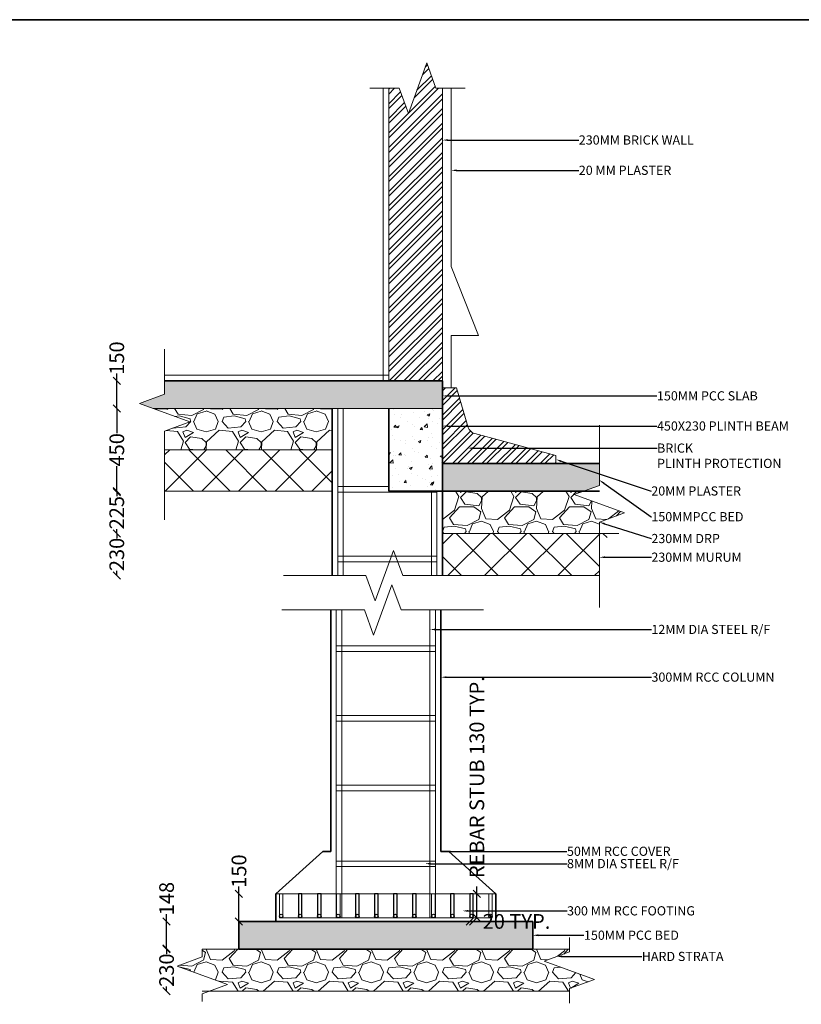
# Model space of a CAD drawing. Units: millimetres. Extents: x -6233 to 6805, y -5269 to 4890.
# Tile 3 of 4: x -1936 to 2321, y -472 to 4890. Entities that reach past the tile are written whole.
import ezdxf
from ezdxf import colors
from ezdxf.entities.mleader import LeaderData, LeaderLine
from ezdxf.math import Vec2, Vec3

# ---------------------------------------------------------------- set-up
doc = ezdxf.new("R2010")
doc.units = ezdxf.units.MM
doc.header["$MEASUREMENT"] = 0
for name, color, linetype, lineweight in [('S-ANNO-DIMS', 2, 'Continuous', 18), ('S-ANNO-TEXT', 3, 'Continuous', 18), ('S-ANNO-TTLB', 7, 'Continuous', 35), ('S-CONC', 7, 'Continuous', 35), ('S-FNDN', 8, 'Continuous', 18), ('S-PATT', 252, 'Continuous', 13), ('S-REIN', 1, 'Continuous', 25)]:
    doc.layers.add(name, color=color, linetype=linetype, lineweight=lineweight)
doc.styles.get("Standard").update_dxf_attribs({"font": 'arial.ttf'})
doc.dimstyles.get("Standard").update_dxf_attribs({"dimtxt": 80, "dimasz": 40, "dimexe": 0.18, "dimexo": 0.0625, "dimgap": 0.09, "dimtad": 0, "dimdec": 0, "dimzin": 0, "dimdsep": 46, "dimtxsty": 'Standard', "dimblk": 'OBLIQUE', "dimcen": 0.09, "dimadec": 0, "dimazin": 0, "dimtfac": 1, "dimtdec": 0, "dimtofl": 0, "dimtmove": 0, "dimatfit": 3, "dimfxl": 1, "dimfxlon": 1, "dimtolj": 1, "dimtzin": 0, "dimarcsym": 0})

# ---------------------------------------------------------------- blocks, each defined once
blk = doc.blocks.new('_Oblique')
at = {"color": 0, "linetype": 'ByBlock', "lineweight": -2}
blk.add_line((-0.5, -0.5), (0.5, 0.5), dxfattribs=at)
blk = doc.blocks.new('*D10')
at = {"layer": 'DEFPOINTS', "color": 0, "transparency": 16777216}
for p in [(-1136.3, -171.5), (-906.1, -171.5), (-906.1, -401.5)]:
    blk.add_point(p, dxfattribs=at)
at = {"layer": 'S-ANNO-DIMS', "color": 0, "lineweight": -2, "transparency": 16777216}
for p, q in [((-1135.3, -171.5), (-1136.5, -171.5)), ((-1136.3, -171.5), (-1136.3, -197.5)), ((-1135.3, -401.5), (-1136.5, -401.5)), ((-1136.3, -401.5), (-1136.3, -375.5))]:
    blk.add_line(p, q, dxfattribs=at)
at = {"layer": 'S-ANNO-DIMS', "color": 0, "lineweight": -2, "transparency": 16777216, "xscale": 40, "yscale": 40, "zscale": 40}
for p, rotation in [((-1136.3, -171.5), 90), ((-1136.3, -401.5), 270)]:
    blk.add_blockref('_Oblique', p, dxfattribs=dict(at, rotation=rotation))
at = {"layer": 'S-ANNO-DIMS', "color": 0, "transparency": 16777216, "insert": (-1136.3, -286.5), "char_height": 80, "attachment_point": 5, "rotation": 90}
blk.add_mtext('\\A1;230', dxfattribs=at)
blk = doc.blocks.new('*D11')
at = {"layer": 'DEFPOINTS', "color": 0, "transparency": 16777216}
for p in [(-1136.3, -21.5), (-742, -21.5), (-742, -169.1)]:
    blk.add_point(p, dxfattribs=at)
at = {"layer": 'S-ANNO-DIMS', "color": 0, "lineweight": -2, "transparency": 16777216}
for p, q in [((-1136.3, -21.5), (-1136.3, 18.5)), ((-1135.3, -21.5), (-1136.5, -21.5)), ((-1136.3, -169.1), (-1136.3, -21.5)), ((-1135.3, -169.1), (-1136.5, -169.1))]:
    blk.add_line(p, q, dxfattribs=at)
at = {"layer": 'S-ANNO-DIMS', "color": 0, "lineweight": -2, "transparency": 16777216, "xscale": 40, "yscale": 40, "zscale": 40}
for p, rotation in [((-1136.3, -21.5), 90), ((-1136.3, -169.1), 270)]:
    blk.add_blockref('_Oblique', p, dxfattribs=dict(at, rotation=rotation))
at = {"layer": 'S-ANNO-DIMS', "color": 0, "transparency": 16777216, "insert": (-1136.3, 103.3), "char_height": 80, "attachment_point": 5, "rotation": 90}
blk.add_mtext('\\A1;148', dxfattribs=at)
blk = doc.blocks.new('*D12')
at = {"layer": 'DEFPOINTS', "color": 0, "transparency": 16777216}
for p in [(-742, 128.5), (-542, 128.5), (-542, -21.5)]:
    blk.add_point(p, dxfattribs=at)
at = {"layer": 'S-ANNO-DIMS', "color": 0, "lineweight": -2, "transparency": 16777216}
for p, q in [((-742, 128.5), (-742, 168.5)), ((-741, 128.5), (-742.2, 128.5)), ((-742, -21.5), (-742, 128.5)), ((-741, -21.5), (-742.2, -21.5))]:
    blk.add_line(p, q, dxfattribs=at)
at = {"layer": 'S-ANNO-DIMS', "color": 0, "lineweight": -2, "transparency": 16777216, "xscale": 40, "yscale": 40, "zscale": 40}
for p, rotation in [((-742, 128.5), 90), ((-742, -21.5), 270)]:
    blk.add_blockref('_Oblique', p, dxfattribs=dict(at, rotation=rotation))
at = {"layer": 'S-ANNO-DIMS', "color": 0, "transparency": 16777216, "insert": (-742, 253.1), "char_height": 80, "attachment_point": 5, "rotation": 90}
blk.add_mtext('\\A1;150', dxfattribs=at)
blk = doc.blocks.new('*D13')
at = {"layer": 'DEFPOINTS', "color": 0, "transparency": 16777216}
for p in [(-1407.6, 2092.6), (374.4, 2092.6), (374.4, 1862.6)]:
    blk.add_point(p, dxfattribs=at)
at = {"layer": 'S-ANNO-DIMS', "color": 0, "lineweight": -2, "transparency": 16777216}
for p, q in [((-1406.6, 2092.6), (-1407.8, 2092.6)), ((-1407.6, 2092.6), (-1407.6, 2066.7)), ((-1407.6, 1862.6), (-1407.6, 1888.6)), ((-1406.6, 1862.6), (-1407.8, 1862.6))]:
    blk.add_line(p, q, dxfattribs=at)
at = {"layer": 'S-ANNO-DIMS', "color": 0, "lineweight": -2, "transparency": 16777216, "xscale": 40, "yscale": 40, "zscale": 40}
for p, rotation in [((-1407.6, 2092.6), 90), ((-1407.6, 1862.6), 270)]:
    blk.add_blockref('_Oblique', p, dxfattribs=dict(at, rotation=rotation))
at = {"layer": 'S-ANNO-DIMS', "color": 0, "transparency": 16777216, "insert": (-1407.6, 1977.6), "char_height": 80, "attachment_point": 5, "rotation": 90}
blk.add_mtext('\\A1;230', dxfattribs=at)
blk = doc.blocks.new('*D14')
at = {"layer": 'DEFPOINTS', "color": 0, "transparency": 16777216}
for p in [(-1407.8, 2317.5), (366.2, 2317.5), (366.2, 2092.6)]:
    blk.add_point(p, dxfattribs=at)
at = {"layer": 'S-ANNO-DIMS', "color": 0, "lineweight": -2, "transparency": 16777216}
for p, q in [((-1406.8, 2317.5), (-1408, 2317.5)), ((-1407.8, 2317.5), (-1407.8, 2294.5)), ((-1406.8, 2092.6), (-1408, 2092.6)), ((-1407.8, 2092.6), (-1407.8, 2115.6))]:
    blk.add_line(p, q, dxfattribs=at)
at = {"layer": 'S-ANNO-DIMS', "color": 0, "lineweight": -2, "transparency": 16777216, "xscale": 40, "yscale": 40, "zscale": 40}
for p, rotation in [((-1407.8, 2317.5), 90), ((-1407.8, 2092.6), 270)]:
    blk.add_blockref('_Oblique', p, dxfattribs=dict(at, rotation=rotation))
at = {"layer": 'S-ANNO-DIMS', "color": 0, "transparency": 16777216, "insert": (-1407.8, 2205), "char_height": 80, "attachment_point": 5, "rotation": 90}
blk.add_mtext('\\A1;225', dxfattribs=at)
blk = doc.blocks.new('*D15')
at = {"layer": 'DEFPOINTS', "color": 0, "transparency": 16777216}
for p in [(-1407.4, 2772.6), (-1147, 2772.6), (-1147, 2322.6)]:
    blk.add_point(p, dxfattribs=at)
at = {"layer": 'S-ANNO-DIMS', "color": 0, "lineweight": -2, "transparency": 16777216}
for p, q in [((-1406.4, 2772.6), (-1407.6, 2772.6)), ((-1407.4, 2772.6), (-1407.4, 2637.6)), ((-1407.4, 2322.6), (-1407.4, 2457.7)), ((-1406.4, 2322.6), (-1407.6, 2322.6))]:
    blk.add_line(p, q, dxfattribs=at)
at = {"layer": 'S-ANNO-DIMS', "color": 0, "lineweight": -2, "transparency": 16777216, "xscale": 40, "yscale": 40, "zscale": 40}
for p, rotation in [((-1407.4, 2772.6), 90), ((-1407.4, 2322.6), 270)]:
    blk.add_blockref('_Oblique', p, dxfattribs=dict(at, rotation=rotation))
at = {"layer": 'S-ANNO-DIMS', "color": 0, "transparency": 16777216, "insert": (-1407.4, 2547.6), "char_height": 80, "attachment_point": 5, "rotation": 90}
blk.add_mtext('\\A1;450', dxfattribs=at)
blk = doc.blocks.new('*D16')
at = {"layer": 'DEFPOINTS', "color": 0, "transparency": 16777216}
for p in [(-1407.6, 2922.6), (-1113.4, 2922.6), (-1113.4, 2772.6)]:
    blk.add_point(p, dxfattribs=at)
at = {"layer": 'S-ANNO-DIMS', "color": 0, "lineweight": -2, "transparency": 16777216}
for p, q in [((-1407.6, 2922.6), (-1407.6, 2962.6)), ((-1406.6, 2922.6), (-1407.8, 2922.6)), ((-1407.6, 2772.6), (-1407.6, 2922.6)), ((-1406.6, 2772.6), (-1407.8, 2772.6))]:
    blk.add_line(p, q, dxfattribs=at)
at = {"layer": 'S-ANNO-DIMS', "color": 0, "lineweight": -2, "transparency": 16777216, "xscale": 40, "yscale": 40, "zscale": 40}
for p, rotation in [((-1407.6, 2922.6), 90), ((-1407.6, 2772.6), 270)]:
    blk.add_blockref('_Oblique', p, dxfattribs=dict(at, rotation=rotation))
at = {"layer": 'S-ANNO-DIMS', "color": 0, "transparency": 16777216, "insert": (-1407.6, 3047.2), "char_height": 80, "attachment_point": 5, "rotation": 90}
blk.add_mtext('\\A1;150', dxfattribs=at)
blk = doc.blocks.new('REBAR-STUB-TRAP')
for p, q in [((0, 130), (0, 32.5)), ((19.5, 130), (0, 130)), ((19.5, 0), (19.5, 130)), ((0, 32.5), (0, 0))]:
    blk.add_line(p, q)
blk = doc.blocks.new('*D30')
at = {"layer": 'DEFPOINTS', "color": 0, "transparency": 16777216}
for p in [(534.3, 128.5), (553.8, 128.5), (534.3, -1.5)]:
    blk.add_point(p, dxfattribs=at)
at = {"layer": 'S-ANNO-DIMS', "color": 0, "lineweight": -2, "transparency": 16777216}
for p, q in [((553.8, 128.5), (553.8, 168.5)), ((552.8, 128.5), (554, 128.5)), ((553.8, -1.5), (553.8, 128.5)), ((552.8, -1.5), (554, -1.5))]:
    blk.add_line(p, q, dxfattribs=at)
at = {"layer": 'S-ANNO-DIMS', "color": 0, "lineweight": -2, "transparency": 16777216, "xscale": 40, "yscale": 40, "zscale": 40}
for p, rotation in [((553.8, 128.5), 90), ((553.8, -1.5), 270)]:
    blk.add_blockref('_Oblique', p, dxfattribs=dict(at, rotation=rotation))
at = {"layer": 'S-ANNO-DIMS', "color": 0, "transparency": 16777216, "insert": (553.8, 764.9), "char_height": 80, "attachment_point": 5, "rotation": 90}
blk.add_mtext('\\A1;REBAR STUB 130 TYP.', dxfattribs=at)
blk = doc.blocks.new('*D31')
at = {"layer": 'DEFPOINTS', "color": 0, "transparency": 16777216}
for p in [(514.8, -1.5), (534.3, -1.5), (534.3, -21)]:
    blk.add_point(p, dxfattribs=at)
at = {"layer": 'S-ANNO-DIMS', "color": 0, "lineweight": -2, "transparency": 16777216}
for p, q in [((514.8, -20), (514.8, -21.2)), ((514.8, -21), (534.3, -21)), ((534.3, -20), (534.3, -21.2)), ((534.3, -21), (574.3, -21))]:
    blk.add_line(p, q, dxfattribs=at)
at = {"layer": 'S-ANNO-DIMS', "color": 0, "lineweight": -2, "transparency": 16777216, "xscale": 40, "yscale": 40, "zscale": 40, "rotation": 180}
blk.add_blockref('_Oblique', (514.8, -21), dxfattribs=at)
at = {"layer": 'S-ANNO-DIMS', "color": 0, "lineweight": -2, "transparency": 16777216, "xscale": 40, "yscale": 40, "zscale": 40}
blk.add_blockref('_Oblique', (534.3, -21), dxfattribs=at)
at = {"layer": 'S-ANNO-DIMS', "color": 0, "transparency": 16777216, "insert": (769.8, -21), "char_height": 80, "attachment_point": 5}
blk.add_mtext('\\A1;20 TYP.', dxfattribs=at)

msp = doc.modelspace()

# ---------------------------------------------------------------- hatches: boundary and pattern name
at = {"layer": 'S-PATT'}
h = msp.add_hatch(dxfattribs=at)
h.set_pattern_fill('ANSI32', color=256, scale=150)
h.set_pattern_definition([(45, (4232.944, 0), (-39.77476, 39.77476), []), (45, (4259.46, 0), (-39.77476, 39.77476), [])])
h.paths.add_polyline_path([(74, 2922.6), (366.2, 2922.6), (366.2, 4517.1), (331.1, 4517.1), (281.1, 4654.5), (181.1, 4379.8), (131.1, 4517.1), (74, 4517.1)])
h.paths.add_polyline_path([(442.5, 2885.1), (366.2, 2885.1), (366.2, 2472.6), (984.3, 2472.6), (984.3, 2517.5), (542.1, 2636.1, -0.259704), (507.2, 2670)])
h = msp.add_hatch(dxfattribs=at)
h.set_pattern_fill('AR-SAND', color=256, scale=50)
h.set_pattern_definition([(37.5, (-1523.09, 0), (-3.1497, 96.3412), [0, -76, 0, -85, 0, -81.25]), (7.5, (-1523.09, 0), (88.489, 141.1073), [0, -41, 0, -68.5, 0, -26.25]), (327.5, (-1584.59, 0), (155.7071, 0.283), [0, -25, 0, -90, 0, -117.5]), (317.5, (-1584.59, 0), (150.3063, 43.8838), [0, -12.5, 0, -59, 0, -67.5])])
h.paths.add_polyline_path([(-1147, 2922.6), (-1147, 2849.8), (-1284.4, 2799.8), (-1209.9, 2772.6), (-233.8, 2772.6), (366.2, 2772.6), (366.2, 2922.6)])
h.paths.add_polyline_path([(1135.7, 2322.6), (1221, 2353.7), (1221, 2472.6), (366.2, 2472.6), (366.2, 2322.6)])
h.paths.add_polyline_path([(-742, -21.5), (-742, -171.5), (858, -171.5), (858, -21.5)])
h = msp.add_hatch(dxfattribs=at)
h.set_pattern_fill('GRAVEL', color=256, scale=300)
h.set_pattern_definition([(228.0128, (-1307.09, 300), (-2400, -2700), [40.361, -3995.726]), (184.96974, (-1334.09, 270), (3600, 300), [69.26, -6856.7774]), (132.51045, (-1403.09, 264), (3000, -3300), [48.836, -4834.81]), (267.2737, (-1520.09, 189), (300, 6000), [63.071, -6244.067]), (292.83365, (-1523.09, 126), (-1500, 3600), [61.8465, -6122.812]), (357.2737, (-1499.09, 69), (-6000, 300), [63.071, -6244.067]), (37.69424, (-1436.09, 66), (-3900, -3000), [83.409, -8257.4546]), (72.25533, (-1370.09, 117), (2100, 6600), [78.7464, -7795.8964]), (121.42957, (-1346.09, 192), (-2400, 3900), [63.285, -6265.222]), (175.23636, (-1379.09, 246), (3300, -300), [72.25, -3540.229]), (222.39744, (-1451.09, 252), (-3600, -3300), [93.4344, -9250.0125]), (138.8141, (-1223.09, 186), (-2100, 1800), [31.89, -3157.153]), (171.46923, (-1247.09, 207), (3900, -600), [60.671, -6006.453]), (225, (-1307.1, 216), (-3e-14, -300), [42.426, -381.838]), (203.1986, (-1328.09, 252), (1500, 600), [22.847, -2261.885]), (291.8014, (-1349.09, 243), (-300, 900), [32.311, -1583.239]), (30.9638, (-1337.09, 213), (900, 600), [52.479, -1696.807]), (161.565, (-1292.09, 240), (600, -300), [37.947, -910.736]), (16.38954, (-1523.09, 243), (3000, 900), [53.16, -5262.854]), (70.3462, (-1472.09, 258), (-1200, -3300), [44.598, -4415.222]), (293.1986, (-1292.09, 300), (-600, 1500), [45.694, -2239.037]), (343.61046, (-1274.09, 258), (-3000, 900), [53.16, -5262.854]), (339.444, (-1523.09, 57), (-1500, 600), [51.264, -2511.937]), (294.77514, (-1475.09, 39), (-1500, 3300), [42.953, -4252.393]), (66.8014, (-1289.09, 0), (600, 1500), [45.694, -2239.037]), (17.354, (-1271.09, 42), (-3900, -1200), [50.289, -4978.627]), (69.444, (-1436.09, 0), (-600, -1500), [25.632, -2537.569]), (101.31, (-1307.09, 0), (-300, 1200), [15.297, -1514.409]), (165.9638, (-1310.09, 15), (900, -300), [61.846, -1175.085]), (186.009, (-1370.09, 30), (3000, 300), [57.315, -5674.177]), (303.69, (-1337.09, 186), (-300, 600), [43.267, -1038.399]), (353.15723, (-1313.09, 150), (5100, -600), [75.538, -7478.269]), (60.9454, (-1238.09, 141), (-1200, -2100), [30.887, -3057.802]), (90, (-1223.1, 168), (-300, 300), [18, -282]), (120.25644, (-1376.09, 39), (1200, -2100), [41.677, -4126.056]), (48.0128, (-1397.09, 75), (2400, 2700), [80.722, -3955.366]), (0, (-1343.1, 135), (300, 300), [78, -222]), (325.30485, (-1265.09, 135), (3000, -2100), [47.434, -4695.982]), (254.0546, (-1226.09, 108), (-300, -1200), [43.68, -2140.352]), (207.64598, (-1238.09, 66), (-5700, -3000), [71.1195, -7040.842]), (175.42608, (-1301.09, 33), (-3900, 300), [75.24, -7448.722])])
h.paths.add_polyline_path([(-742, -171.5), (-942, -171.5), (-942, -214.6), (-1079.4, -264.6), (-804.6, -364.6), (-906.1, -401.5), (1058, -401.5), (1058, -387.2), (1195.4, -337.2), (920.6, -237.2), (1058, -187.2), (1058, -171.5), (858, -171.5)])
h.paths.add_polyline_path([(366.2, 2322.6), (366.2, 2092.6), (1221, 2092.6), (1221, 2153.7), (1358.4, 2203.7), (1083.6, 2303.7), (1135.7, 2322.6)])
h.paths.add_polyline_path([(-1209.9, 2772.6), (-1009.7, 2699.8), (-1147, 2649.8), (-1147, 2547.6), (-233.8, 2547.6), (-233.8, 2772.6)])
h = msp.add_hatch(dxfattribs=at)
h.set_pattern_fill('AR-CONC', color=256, scale=20)
h.set_pattern_definition([(50, (-1523.09, 0), (143.452, -12.5504), [15, -165]), (355, (-1523.09, 0), (-27.75, 150.4384), [12, -132]), (100.4514, (-1511.14, -1.05), (115.702, 137.888), [12.748, -140.2284]), (46.184, (-1523.09, 40), (213.448, -33.104), [22.5, -247.5]), (96.6356, (-1505.3, 37.24), (186.932, 194.824), [19.122, -210.343]), (351.184, (-1523.1, 40), (186.932, 194.824), [18, -198]), (21, (-1503.09, 30), (119.3814, -80.5238), [15, -165]), (326, (-1503.09, 30), (48.663, 145.03), [12, -132]), (71.4514, (-1493.14, 23.29), (168.0445, 64.506), [12.748, -140.2284]), (37.5, (-1523.09, 0), (2.432, 66.5788), [0, -130.4, 0, -134, 0, -132.5]), (7.5, (-1523.09, 0), (52.6139, 78.8823), [0, -76.4, 0, -127.4, 0, -50.5]), (327.5, (-1567.69, 0), (106.7645, -4.511), [0, -50, 0, -156, 0, -207]), (317.5, (-1587.69, 0), (116.6372, 20.021), [0, -65, 0, -103.6, 0, -147])])
h.paths.add_polyline_path([(74, 2322.6), (366.2, 2322.6), (366.2, 2772.6), (74, 2772.6)])
h = msp.add_hatch(dxfattribs=at)
h.set_pattern_fill('¶À¿×²ÄÁÏ', color=256, scale=50)
h.set_pattern_definition([(45, (4332.94, 0), (-100, 100), []), (135, (4332.94, 0), (-100, -100), [])])
h.paths.add_polyline_path([(-233.8, 2322.6), (-233.8, 2547.6), (-1147, 2547.6), (-1147, 2322.6)])
h.paths.add_polyline_path([(366.2, 2092.6), (366.2, 1862.6), (1221, 1862.6), (1221, 2054.3), (1326.4, 2092.6)])

# ---------------------------------------------------------------- linework, layer by layer
at = {"layer": 'S-ANNO-TTLB'}
msp.add_lwpolyline([(-6232.9, 4890.2), (2600.5, 4890.2), (2600.5, -1330.2), (-6232.9, -1330.2)], close=True, dxfattribs=at)
at = {"layer": 'S-CONC'}
for p, q in [((366.2, 2922.6), (-1147, 2922.6)), ((366.2, 2922.6), (366.2, 1862.6)), ((-233.8, 2772.6), (-233.8, 1862.6)), ((74, 2322.6), (74, 2772.6)), ((366.2, 2472.6), (1221, 2472.6)), ((366.2, 2322.6), (74, 2322.6)), ((366.2, 2322.6), (1221, 2322.6)), ((-242, 360.6), (-242, 1675.2)), ((358, 360.6), (358, 1675.2)), ((-542, 128.5), (-284.6, 360.6)), ((-284.6, 360.6), (-242, 360.6)), ((400.7, 360.6), (358, 360.6)), ((658, 128.5), (400.7, 360.6)), ((-542, -21.5), (-542, 128.5)), ((658, -21.5), (658, 128.5)), ((-742, -21.5), (858, -21.5)), ((-742, -171.5), (-742, -21.5)), ((858, -21.5), (658, -21.5)), ((858, -171.5), (858, -21.5)), ((858, -171.5), (-742, -171.5))]:
    msp.add_line(p, q, dxfattribs=at)
at = {"layer": 'S-FNDN'}
for p, q in [((44, 2922.6), (44, 4517.1)), ((74, 2922.6), (74, 4517.1)), ((366.2, 4517.1), (366.2, 2922.6)), ((413.1, 4517.1), (413.1, 3546.1)), ((413.1, 3546.1), (562.4, 3169.4)), ((562.4, 3169.4), (413.1, 3169.4)), ((413.1, 3169.4), (413.1, 2887.3)), ((74, 2954.4), (-1147, 2954.4)), ((442.5, 2885.1), (366.2, 2885.1)), ((442.5, 2885.1), (507.2, 2670)), ((-233.8, 2772.6), (-1209.9, 2772.6)), ((-233.8, 2772.6), (366.2, 2772.6)), ((-203.8, 1862.6), (-203.8, 2772.6)), ((-173.8, 1862.6), (-173.8, 2772.6)), ((542.1, 2636.1), (984.3, 2517.5)), ((-233.8, 2547.6), (-1147, 2547.6)), ((984.3, 2517.5), (984.3, 2472.6)), ((-233.8, 2322.6), (-1147, 2322.6)), ((-203.8, 2347.5), (74, 2347.5)), ((-203.8, 2317.5), (336.2, 2317.5)), ((306.2, 1862.6), (306.2, 2322.6)), ((336.2, 1862.6), (336.2, 2322.6)), ((366.2, 2092.6), (1326.4, 2092.6)), ((-203.8, 1967.6), (336.2, 1967.6)), ((-203.8, 1937.6), (336.2, 1937.6)), ((366.2, 1862.6), (1221, 1862.6)), ((-212, -1.5), (-212, 1675.2)), ((-182, -1.5), (-182, 1675.2)), ((298, -1.5), (298, 1675.2)), ((328, -1.5), (328, 1675.2)), ((-212, 1479.8), (328, 1479.8)), ((-212, 1449.8), (328, 1449.8)), ((-212, 1100), (328, 1100)), ((-212, 1070), (328, 1070)), ((-212, 720.2), (328, 720.2)), ((-212, 690.2), (328, 690.2)), ((-212, 307.7), (328, 307.7)), ((-212, 277.7), (328, 277.7)), ((-542, 128.5), (658, 128.5)), ((-522, 128.5), (-522, 31)), ((-502.5, 128.5), (-522, 128.5)), ((-502.5, -1.5), (-502.5, 128.5)), ((-210.9, 128.5), (-210.9, 31)), ((-191.4, 128.5), (-210.9, 128.5)), ((-191.4, -1.5), (-191.4, 128.5)), ((307.5, 128.5), (307.5, 31)), ((327, 128.5), (307.5, 128.5)), ((327, -1.5), (327, 128.5)), ((618.5, 128.5), (618.5, 31)), ((638, 128.5), (618.5, 128.5)), ((638, -1.5), (638, 128.5)), ((-522, 31), (-522, -1.5)), ((-210.9, 31), (-210.9, -1.5)), ((307.5, 31), (307.5, -1.5)), ((618.5, 31), (618.5, -1.5)), ((-742, -21.5), (-542, -21.5)), ((-522, -1.5), (638, -1.5)), ((-742, -171.5), (-942, -171.5)), ((858, -171.5), (1058, -171.5)), ((-942, -401.5), (1058, -401.5))]:
    msp.add_line(p, q, dxfattribs=at)
for points in [[(-28.6, 4517.1), (131.1, 4517.1), (181.1, 4379.8), (281.1, 4654.5), (331.1, 4517.1), (490.8, 4517.1)], [(-1147, 3096.1), (-1147, 2849.8), (-1284.4, 2799.8), (-1009.7, 2699.8), (-1147, 2649.8), (-1147, 2165.5)], [(1221, 2681.1), (1221, 2353.7), (1083.6, 2303.7), (1358.4, 2203.7), (1221, 2153.7), (1221, 1689.6)], [(-499.7, 1862.6), (-50.3, 1862.6), (-0.3, 1725.3), (99.7, 2000), (149.7, 1862.6), (599.1, 1862.6)], [(-507.7, 1675.2), (-58.5, 1675.2), (-8.5, 1537.8), (91.5, 1812.6), (141.5, 1675.2), (590.8, 1675.2)], [(1058, -108.7), (1058, -187.2), (920.6, -237.2), (1195.4, -337.2), (1058, -387.2), (1058, -465.6)], [(-942, -171.3), (-942, -214.6), (-1079.4, -264.6), (-804.6, -364.6), (-942, -414.6), (-942, -457.8)]]:
    msp.add_lwpolyline(points, dxfattribs=at)
msp.add_arc((555.1, 2684.4), 50, 196.7477, 254.9811, dxfattribs=at)
at = {"layer": 'S-REIN'}
for centre in [(-512.2, 8.3), (-408.6, 8.3), (-304.9, 8.3), (-201.2, 8.3), (-97.5, 8.3), (6.2, 8.3), (109.9, 8.3), (213.5, 8.3), (317.2, 8.3), (420.9, 8.3), (524.6, 8.3), (628.3, 8.3)]:
    msp.add_circle(centre, 9.75, dxfattribs=at)

# ---------------------------------------------------------------- block references
for p in [(-418.3, -1.5), (-314.6, -1.5), (-107.3, -1.5), (-3.6, -1.5), (100.1, -1.5), (203.8, -1.5), (411.1, -1.5), (514.8, -1.5)]:
    msp.add_blockref('REBAR-STUB-TRAP', p, dxfattribs=at)

# ---------------------------------------------------------------- dimensions: what is measured, and where the dimension line sits
at = {"layer": 'S-ANNO-DIMS'}
for base, p1, p2, picture, middle in [((-1407.6, 2922.6), (-1113.4, 2772.6), (-1113.4, 2922.6), '*D16', (-1407.6, 3047.2)), ((-1407.4, 2772.6), (-1147, 2322.6), (-1147, 2772.6), '*D15', (-1407.4, 2547.6)), ((-1407.8, 2317.5), (366.2, 2092.6), (366.2, 2317.5), '*D14', (-1407.8, 2205)), ((-1407.6, 2092.6), (374.4, 1862.6), (374.4, 2092.6), '*D13', (-1407.6, 1977.6)), ((-742, 128.5), (-542, -21.5), (-542, 128.5), '*D12', (-742, 253.1)), ((-1136.3, -21.5), (-742, -169.1), (-742, -21.5), '*D11', (-1136.3, 103.3)), ((-1136.3, -171.5), (-906.1, -401.5), (-906.1, -171.5), '*D10', (-1136.3, -286.5))]:
    dim = msp.add_linear_dim(base=base, p1=p1, p2=p2, angle=90, dimstyle='Standard', override={"dimclrd": 0, "dimclre": 0, "dimclrt": 0}, dxfattribs=at)
    dim.commit()
    dim.dimension.update_dxf_attribs({"geometry": picture, "text_midpoint": middle})
dim = msp.add_linear_dim(base=(553.8, 128.5), p1=(534.3, -1.5), p2=(534.3, 128.5), angle=90, text='REBAR STUB <> TYP.', dimstyle='Standard', override={"dimdec": 0, "dimrnd": 0, "dimzin": 0, "dimlunit": 2}, dxfattribs=at)
dim.commit()
dim.dimension.update_dxf_attribs({"geometry": '*D30', "text_midpoint": (553.8, 764.9)})
dim = msp.add_linear_dim(base=(534.3296935, -20.9919267), p1=(514.8296935, -1.4919267), p2=(534.3296935, -1.4919267), text='<> TYP.', dimstyle='Standard', override={"dimdec": 0, "dimrnd": 0, "dimzin": 0, "dimlunit": 2}, dxfattribs=at)
dim.commit()
dim.dimension.update_dxf_attribs({"geometry": '*D31', "text_midpoint": (769.8085066, -20.9919267)})

# ---------------------------------------------------------------- leaders
at = {"layer": 'S-ANNO-TEXT'}
ml = msp.add_multileader_mtext('Standard', dxfattribs=at)
ml.set_content('230MM BRICK WALL', color=256)
ml.set_leader_properties()
ml.build(insert=Vec2(0, 0))
ml.multileader.update_dxf_attribs({"dogleg_length": 0.36, "arrow_head_size": 30})
ctx = ml.context
ctx.base_point, ctx.char_height, ctx.arrow_head_size, ctx.landing_gap_size, ctx.plane_origin = Vec3(1109, 4234.6), 50, 30, 0.09, Vec3(366.2, 4234.6)
notes = []
notes.append((ctx, [(0, (1, 1, 0), (1108.6, 4234.6), (1, 0), 0.36, [(0, [(366.2, 4234.6)], 0, [])])]))
ctx.mtext.insert, ctx.mtext.flow_direction = Vec3(1109.1, 4260), 5
ml = msp.add_multileader_mtext('Standard', dxfattribs=at)
ml.set_content('20 MM PLASTER', color=256)
ml.set_leader_properties()
ml.build(insert=Vec2(0, 0))
ml.multileader.update_dxf_attribs({"dogleg_length": 0.36, "arrow_head_size": 30})
ctx = ml.context
ctx.base_point, ctx.char_height, ctx.arrow_head_size, ctx.landing_gap_size, ctx.plane_origin = Vec3(1109, 4069.6), 50, 30, 0.09, Vec3(413.1, 4069.6)
notes.append((ctx, [(0, (1, 1, 0), (1108.6, 4069.6), (1, 0), 0.36, [(0, [(413.1, 4069.6)], 0, [])])]))
ctx.mtext.insert, ctx.mtext.flow_direction = Vec3(1109.1, 4095), 5
ml = msp.add_multileader_mtext('Standard', dxfattribs=at)
ml.set_content('150MM PCC SLAB', color=256)
ml.set_leader_properties()
ml.build(insert=Vec2(0, 0))
ml.multileader.update_dxf_attribs({"dogleg_length": 0.36, "arrow_head_size": 30})
ctx = ml.context
ctx.base_point, ctx.char_height, ctx.arrow_head_size, ctx.landing_gap_size, ctx.plane_origin = Vec3(1534.9, 2841.1), 50, 30, 0.09, Vec3(366.2, 2841.1)
notes.append((ctx, [(0, (1, 1, 0), (1534.5, 2841.1), (1, 0), 0.36, [(0, [(366.2, 2841.1)], 0, [])])]))
ctx.mtext.insert, ctx.mtext.flow_direction = Vec3(1535, 2866.5), 5
ml = msp.add_multileader_mtext('Standard', dxfattribs=at)
ml.set_content('450X230 PLINTH BEAM', color=256)
ml.set_leader_properties()
ml.build(insert=Vec2(0, 0))
ml.multileader.update_dxf_attribs({"dogleg_length": 0.36, "arrow_head_size": 30})
ctx = ml.context
ctx.base_point, ctx.char_height, ctx.arrow_head_size, ctx.landing_gap_size, ctx.plane_origin = Vec3(1534.9, 2677), 50, 30, 0.09, Vec3(366.2, 2677)
notes.append((ctx, [(0, (1, 1, 0), (1534.5, 2677), (1, 0), 0.36, [(0, [(366.2, 2677)], 0, [])])]))
ctx.mtext.insert, ctx.mtext.flow_direction = Vec3(1535, 2702.4), 5
ml = msp.add_multileader_mtext('Standard', dxfattribs=at)
ml.set_content('BRICK\\PPLINTH PROTECTION', color=256)
ml.set_leader_properties()
ml.build(insert=Vec2(0, 0))
ml.multileader.update_dxf_attribs({"dogleg_length": 0.36, "arrow_head_size": 30})
ctx = ml.context
ctx.base_point, ctx.char_height, ctx.arrow_head_size, ctx.landing_gap_size, ctx.plane_origin = Vec3(1535.3, 2556.6), 50, 30, 0.09, Vec3(504.3, 2556.6)
notes.append((ctx, [(0, (1, 1, 0), (1535, 2556.6), (1, 0), 0.36, [(0, [(504.3, 2556.6)], 0, [])])]))
ctx.mtext.insert, ctx.mtext.flow_direction = Vec3(1535.4, 2582), 5
ml = msp.add_multileader_mtext('Standard', dxfattribs=at)
ml.set_content('20MM PLASTER', color=256)
ml.set_leader_properties()
ml.build(insert=Vec2(0, 0))
ml.multileader.update_dxf_attribs({"dogleg_length": 0.36, "arrow_head_size": 30})
ctx = ml.context
ctx.base_point, ctx.char_height, ctx.arrow_head_size, ctx.landing_gap_size, ctx.plane_origin = Vec3(1504, 2323.2), 50, 30, 0.09, Vec3(984.3, 2495.1)
notes.append((ctx, [(0, (1, 1, 0), (1503.7, 2323.2), (1, 0), 0.36, [(0, [(984.3, 2495.1)], 0, [])])]))
ctx.mtext.insert, ctx.mtext.flow_direction = Vec3(1504.1, 2348.6), 5
ml = msp.add_multileader_mtext('Standard', dxfattribs=at)
ml.set_content('150MMPCC BED', color=256)
ml.set_leader_properties()
ml.build(insert=Vec2(0, 0))
ml.multileader.update_dxf_attribs({"dogleg_length": 0.36, "arrow_head_size": 30})
ctx = ml.context
ctx.base_point, ctx.char_height, ctx.arrow_head_size, ctx.landing_gap_size, ctx.plane_origin = Vec3(1504.4, 2182.9), 50, 30, 0.09, Vec3(1221, 2382.9)
notes.append((ctx, [(0, (1, 1, 0), (1504, 2182.9), (1, 0), 0.36, [(0, [(1221, 2382.9)], 0, [])])]))
ctx.mtext.insert, ctx.mtext.flow_direction = Vec3(1504.5, 2208.3), 5
ml = msp.add_multileader_mtext('Standard', dxfattribs=at)
ml.set_content('230MM DRP', color=256)
ml.set_leader_properties()
ml.build(insert=Vec2(0, 0))
ml.multileader.update_dxf_attribs({"dogleg_length": 0.36, "arrow_head_size": 30})
ctx = ml.context
ctx.base_point, ctx.char_height, ctx.arrow_head_size, ctx.landing_gap_size, ctx.plane_origin = Vec3(1504.4, 2063.9), 50, 30, 0.09, Vec3(1221, 2153.7)
notes.append((ctx, [(0, (1, 1, 0), (1504, 2063.9), (1, 0), 0.36, [(0, [(1221, 2153.7)], 0, [])])]))
ctx.mtext.insert, ctx.mtext.flow_direction = Vec3(1504.5, 2089.4), 5
ml = msp.add_multileader_mtext('Standard', dxfattribs=at)
ml.set_content('230MM MURUM', color=256)
ml.set_leader_properties()
ml.build(insert=Vec2(0, 0))
ml.multileader.update_dxf_attribs({"dogleg_length": 0.36, "arrow_head_size": 30})
ctx = ml.context
ctx.base_point, ctx.char_height, ctx.arrow_head_size, ctx.landing_gap_size, ctx.plane_origin = Vec3(1504.4, 1962.4), 50, 30, 0.09, Vec3(1221, 1962.4)
notes.append((ctx, [(0, (1, 1, 0), (1504, 1962.4), (1, 0), 0.36, [(0, [(1221, 1962.4)], 0, [])])]))
ctx.mtext.insert, ctx.mtext.flow_direction = Vec3(1504.5, 1987.8), 5
ml = msp.add_multileader_mtext('Standard', dxfattribs=at)
ml.set_content('12MM DIA STEEL R/F', color=256)
ml.set_leader_properties()
ml.build(insert=Vec2(0, 0))
ml.multileader.update_dxf_attribs({"dogleg_length": 0.36, "arrow_head_size": 30})
ctx = ml.context
ctx.base_point, ctx.char_height, ctx.arrow_head_size, ctx.landing_gap_size, ctx.plane_origin = Vec3(1504.4, 1568.9), 50, 30, 0.09, Vec3(298, 1568.9)
notes.append((ctx, [(0, (1, 1, 0), (1504, 1568.9), (1, 0), 0.36, [(0, [(298, 1568.9)], 0, [])])]))
ctx.mtext.insert, ctx.mtext.flow_direction = Vec3(1504.5, 1594.3), 5
ml = msp.add_multileader_mtext('Standard', dxfattribs=at)
ml.set_content('300MM RCC COLUMN ', color=256)
ml.set_leader_properties()
ml.build(insert=Vec2(0, 0))
ml.multileader.update_dxf_attribs({"dogleg_length": 0.36, "arrow_head_size": 30})
ctx = ml.context
ctx.base_point, ctx.char_height, ctx.arrow_head_size, ctx.landing_gap_size, ctx.plane_origin = Vec3(1504.8, 1309), 50, 30, 0.09, Vec3(358, 1309)
notes.append((ctx, [(0, (1, 1, 0), (1504.5, 1309), (1, 0), 0.36, [(0, [(358, 1309)], 0, [])])]))
ctx.mtext.insert, ctx.mtext.flow_direction = Vec3(1504.9, 1334.5), 5
ml = msp.add_multileader_mtext('Standard', dxfattribs=at)
ml.set_content('50MM RCC COVER', color=256)
ml.set_leader_properties()
ml.build(insert=Vec2(0, 0))
ml.multileader.update_dxf_attribs({"dogleg_length": 0.36, "arrow_head_size": 30})
ctx = ml.context
ctx.base_point, ctx.char_height, ctx.arrow_head_size, ctx.landing_gap_size, ctx.plane_origin = Vec3(1044.5, 360.6), 50, 30, 0.09, Vec3(379.3, 360.6)
notes.append((ctx, [(0, (1, 1, 0), (1044.1, 360.6), (1, 0), 0.36, [(0, [(379.3, 360.6)], 0, [])])]))
ctx.mtext.insert, ctx.mtext.flow_direction = Vec3(1044.6, 386), 5
ml = msp.add_multileader_mtext('Standard', dxfattribs=at)
ml.set_content('8MM DIA STEEL R/F', color=256)
ml.set_leader_properties()
ml.build(insert=Vec2(0, 0))
ml.multileader.update_dxf_attribs({"dogleg_length": 0.36, "arrow_head_size": 30})
ctx = ml.context
ctx.base_point, ctx.char_height, ctx.arrow_head_size, ctx.landing_gap_size, ctx.plane_origin = Vec3(1044.8, 293.5), 50, 30, 0.09, Vec3(271.4, 293.5)
notes.append((ctx, [(0, (1, 1, 0), (1044.5, 293.5), (1, 0), 0.36, [(0, [(271.4, 293.5)], 0, [])])]))
ctx.mtext.insert, ctx.mtext.flow_direction = Vec3(1044.9, 319), 5
ml = msp.add_multileader_mtext('Standard', dxfattribs=at)
ml.set_content('300 MM RCC FOOTING', color=256)
ml.set_leader_properties()
ml.build(insert=Vec2(0, 0))
ml.multileader.update_dxf_attribs({"dogleg_length": 0.36, "arrow_head_size": 30})
ctx = ml.context
ctx.base_point, ctx.char_height, ctx.arrow_head_size, ctx.landing_gap_size, ctx.plane_origin = Vec3(1045.2, 36.3), 50, 30, 0.09, Vec3(475.5, 36.3)
notes.append((ctx, [(0, (1, 1, 0), (1044.8, 36.3), (1, 0), 0.36, [(0, [(475.5, 36.3)], 0, [])])]))
ctx.mtext.insert, ctx.mtext.flow_direction = Vec3(1045.3, 61.7), 5
ml = msp.add_multileader_mtext('Standard', dxfattribs=at)
ml.set_content('150MM PCC BED', color=256)
ml.set_leader_properties()
ml.build(insert=Vec2(0, 0))
ml.multileader.update_dxf_attribs({"dogleg_length": 0.36, "arrow_head_size": 30})
ctx = ml.context
ctx.base_point, ctx.char_height, ctx.arrow_head_size, ctx.landing_gap_size, ctx.plane_origin = Vec3(1137.2, -96.5), 50, 30, 0.09, Vec3(858, -96.5)
notes.append((ctx, [(0, (1, 1, 0), (1136.9, -96.5), (1, 0), 0.36, [(0, [(858, -96.5)], 0, [])])]))
ctx.mtext.insert, ctx.mtext.flow_direction = Vec3(1137.3, -71.1), 5
ml = msp.add_multileader_mtext('Standard', dxfattribs=at)
ml.set_content('HARD STRATA', color=256)
ml.set_leader_properties()
ml.build(insert=Vec2(0, 0))
ml.multileader.update_dxf_attribs({"dogleg_length": 0.36, "arrow_head_size": 30})
ctx = ml.context
ctx.base_point, ctx.char_height, ctx.arrow_head_size, ctx.landing_gap_size, ctx.plane_origin = Vec3(1452.1, -212.2), 50, 30, 0.09, Vec3(989.3, -212.2)
notes.append((ctx, [(0, (1, 1, 0), (1451.7, -212.2), (1, 0), 0.36, [(0, [(989.3, -212.2)], 0, [])])]))
ctx.mtext.insert, ctx.mtext.flow_direction = Vec3(1452.2, -186.7), 5
for ctx, leaders in notes:
    for number, flags, end, landing, length, lines in leaders:
        leader = LeaderData()
        leader.index, (leader.has_last_leader_line, leader.has_dogleg_vector, leader.attachment_direction) = number, flags
        leader.last_leader_point, leader.dogleg_vector, leader.dogleg_length = Vec3(end), Vec3(landing), length
        for number, points, colour, breaks in lines:
            line = LeaderLine()
            line.index, line.vertices, line.color, line.breaks = number, Vec3.list(points), colors.encode_raw_color(colour), breaks
            leader.lines.append(line)
        ctx.leaders.append(leader)

doc.saveas('drawing.dxf')
